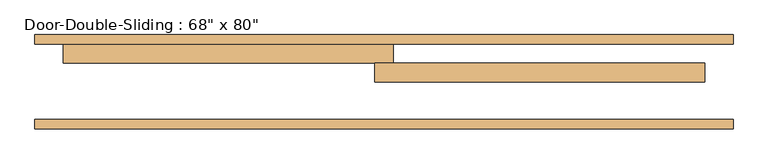
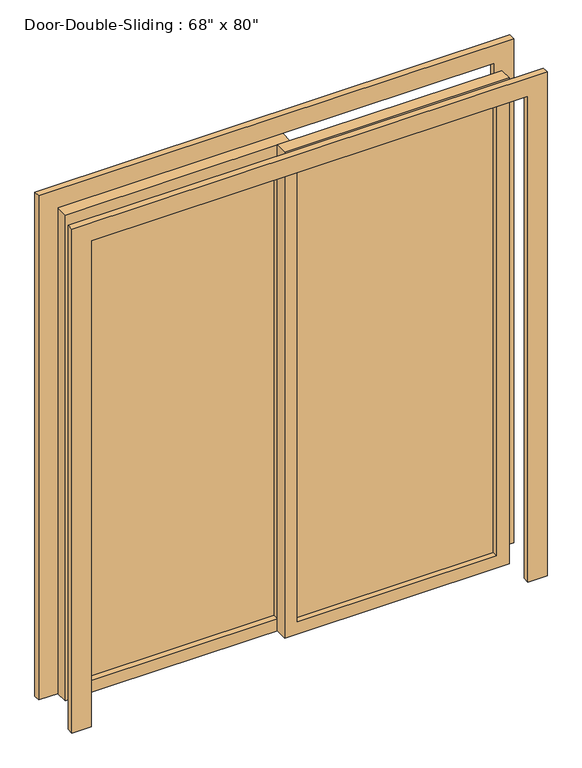
"""IFC4 building model written with IfcOpenShell, lengths in millimetres: door geometry."""

from ifc_helpers import new_model, si_unit, frame, origin, place, context, project, spatial, polyline, outline, extrude, source, transform, mapped, element, save


def door_076b30e0(model_context):
    return source(origin(), model_context, "Body", "SweptSolid", [
        extrude(outline(polyline([(0.0, -939.8), (0.0, -863.6), (2032.0, -863.6), (2032.0, 863.6), (0.0, 863.6), (0.0, 939.8), (2108.2, 939.8), (2108.2, -939.8), (0.0, -939.8)])), frame((0.0, 0.0, 0.0), z_axis=(0.0, 1.0, 0.0), x_axis=(0.0, 0.0, 1.0)), (0.0, 0.0, 1.0), 25.4),
        extrude(outline(polyline([(0.0, 939.8), (2108.2, 939.8), (2108.2, -939.8), (0.0, -939.8), (0.0, -863.6), (2032.0, -863.6), (2032.0, 863.6), (0.0, 863.6), (0.0, 939.8)])), frame((0.0, 228.6, 0.0), z_axis=(0.0, 1.0, 0.0), x_axis=(0.0, 0.0, 1.0)), (0.0, 0.0, 1.0), 25.4),
        extrude(outline(polyline([(2032.0, -25.4), (0.0, -25.4), (0.0, 863.6), (2032.0, 863.6), (2032.0, -25.4)]), holes=[polyline([(1981.2, 25.4), (1981.2, 812.8), (50.8, 812.8), (50.8, 25.4), (1981.2, 25.4)])]), frame((0.0, 127.0, 0.0), z_axis=(0.0, 1.0, 0.0), x_axis=(0.0, 0.0, 1.0)), (0.0, 0.0, 1.0), 50.8),
        extrude(outline(polyline([(2032.0, 25.4), (2032.0, -863.6), (0.0, -863.6), (0.0, 25.4), (2032.0, 25.4)]), holes=[polyline([(1981.2, -25.4), (50.8, -25.4), (50.8, -812.8), (1981.2, -812.8), (1981.2, -25.4)])]), frame((0.0, 177.8, 0.0), z_axis=(0.0, 1.0, 0.0), x_axis=(0.0, 0.0, 1.0)), (0.0, 0.0, 1.0), 50.8),
        extrude(outline(polyline([(25.4, 155.575), (812.8, 155.575), (812.8, 149.225), (25.4, 149.225), (25.4, 155.575)])), frame((0.0, 0.0, 50.8), z_axis=(0.0, 0.0, 1.0), x_axis=(1.0, 0.0, 0.0)), (0.0, 0.0, 1.0), 1930.4),
        extrude(outline(polyline([(-25.4, 200.025), (-812.8, 200.025), (-812.8, 206.375), (-25.4, 206.375), (-25.4, 200.025)])), frame((0.0, 0.0, 50.8), z_axis=(0.0, 0.0, 1.0), x_axis=(1.0, 0.0, 0.0)), (0.0, 0.0, 1.0), 1930.4),
    ])


if __name__ == "__main__":
    model = new_model("IFC4")
    model_context = context("Model", 3, world=origin())
    ifc_project = project(units=[si_unit("LENGTHUNIT", "METRE", prefix="MILLI")], contexts=[model_context])
    site = spatial("IfcSite", under=ifc_project)
    building = spatial("IfcBuilding", under=site)
    placement = place(None, origin())
    door_shape = door_076b30e0(model_context)
    element("IfcDoor", 1, ObjectType="Door-Double-Sliding : 68\" x 80\"", at=placement, inside=building, context=model_context, shape_type="MappedRepresentation", body=[
        mapped(door_shape, transform((0.0, 0.0, 0.0), x_axis=(1.0, 0.0, 0.0), y_axis=(0.0, 1.0, 0.0), z_axis=(0.0, 0.0, 1.0))),
    ])
    save(model, "model.ifc")

# Revit data of these elements
# Type "Door-Double-Sliding : 68\" x 80\""
#   Type Mark = "11"
#   Construction Type Id = "opn-d45"
#   Assembly Code = "C1020"
#   Analytic Construction = "Wood frame, double glass door "
#   Thickness = 0' - 2"
#   Thermal Resistance (R) = 1.8150 (h·ft²·°F)/BTU
#   Heat Transfer Coefficient (U) = 0.5510 BTU/(h·ft²·°F)
#   Height = 6' - 8"
#   Rail Width = 0' - 2"
#   Stiles = 0' - 2"
#   Trim Projection Ext = 0' - 1"
#   Trim Projection Int = 0' - 1"
#   Trim Width = 0' - 3"
#   Width = 5' - 8"
#   Define Thermal Properties by = 1
#   Glazing = Glass
#   Panel Material = Wood - Birch - Solid Stained Light Low Gloss
#   Trim Material = Paint - Sienna
#   Visual Light Transmittance = 0
#   Solar Heat Gain Coefficient = 0
#   Function = (empty or 0)
#   Wall Closure = (empty or 0)
# Element 1 (IfcDoor, "Door-Double-Sliding : 68\" x 80\"")
#   Materials on its faces: "Paint - Sienna", "Wood - Birch - Solid Stained Light Low Gloss", "Glass"
# Materials
#   "Glass": class "Glass", colour RGB 0 128 192, transparency 0.75, Description = "Soda Lime Glass", Cost = 0
#   "Wood - Birch - Solid Stained Light Low Gloss": class "Wood", colour RGB 210 159 95, transparency 0, Cost = 0
#   "Paint - Sienna": colour RGB 118 70 51, transparency 0, Cost = 0
